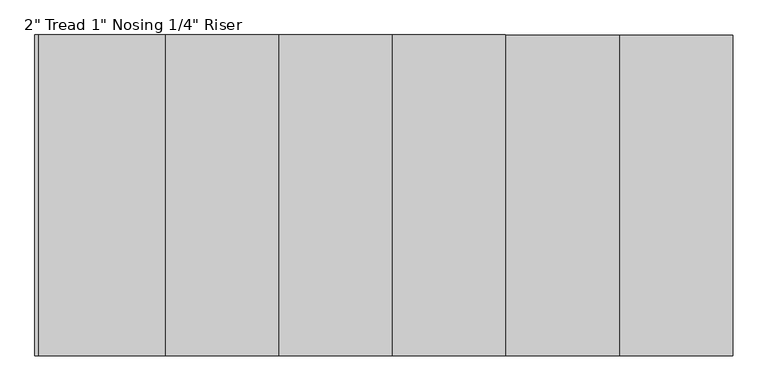
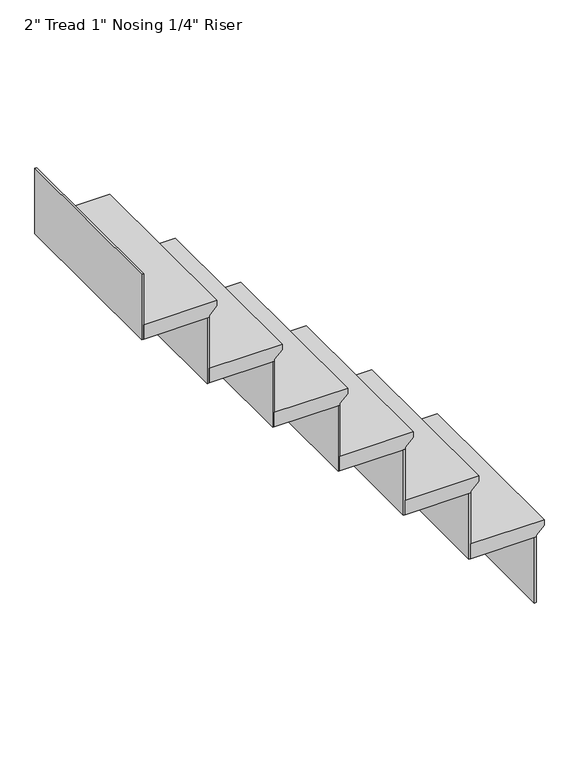
"""IFC4 building model written with IfcOpenShell, lengths in millimetres: stair flight geometry."""

from ifc_helpers import new_model, si_unit, frame, origin, place, context, project, spatial, polyline, outline, extrude, source, transform, mapped, element, save


def stair_flight_92f8819d(model_context):
    return source(origin(), model_context, "Body", "SweptSolid", [
        extrude(outline(polyline([(8229.6, -3732.7409298), (8229.6, -3974.0409298), (8178.8, -3974.0409298), (8178.8, -3758.1409298), (8185.15, -3758.1409298), (8210.55, -3732.7409298), (8229.6, -3732.7409298)])), frame((0.0, -4554.9664375, 0.0), z_axis=(0.0, 1.0, 0.0), x_axis=(0.0, 0.0, 1.0)), (0.0, 0.0, 1.0), 609.6),
        extrude(outline(polyline([(-3764.4909298, -3945.3664375), (-3758.1409298, -3945.3664375), (-3758.1409298, -4554.9664375), (-3764.4909298, -4554.9664375), (-3764.4909298, -3945.3664375)])), frame((0.0, 0.0, 7950.2), z_axis=(0.0, 0.0, 1.0), x_axis=(1.0, 0.0, 0.0)), (0.0, 0.0, 1.0), 228.6),
        extrude(outline(polyline([(-3980.3909298, -3945.3664375), (-3974.0409298, -3945.3664375), (-3974.0409298, -4554.9664375), (-3980.3909298, -4554.9664375), (-3980.3909298, -3945.3664375)])), frame((0.0, 0.0, 8178.8), z_axis=(0.0, 0.0, 1.0), x_axis=(1.0, 0.0, 0.0)), (0.0, 0.0, 1.0), 228.6),
        extrude(outline(polyline([(8458.2, -3948.6409298), (8458.2, -4189.9409298), (8407.4, -4189.9409298), (8407.4, -3974.0409298), (8413.75, -3974.0409298), (8439.15, -3948.6409298), (8458.2, -3948.6409298)])), frame((0.0, -4554.9664375, 0.0), z_axis=(0.0, 1.0, 0.0), x_axis=(0.0, 0.0, 1.0)), (0.0, 0.0, 1.0), 609.6),
        extrude(outline(polyline([(-4196.2909298, -3945.3664375), (-4189.9409298, -3945.3664375), (-4189.9409298, -4554.9664375), (-4196.2909298, -4554.9664375), (-4196.2909298, -3945.3664375)])), frame((0.0, 0.0, 8407.4), z_axis=(0.0, 0.0, 1.0), x_axis=(1.0, 0.0, 0.0)), (0.0, 0.0, 1.0), 228.6),
        extrude(outline(polyline([(8686.8, -4164.5409298), (8686.8, -4405.8409298), (8636.0, -4405.8409298), (8636.0, -4189.9409298), (8642.35, -4189.9409298), (8667.75, -4164.5409298), (8686.8, -4164.5409298)])), frame((0.0, -4554.9664375, 0.0), z_axis=(0.0, 1.0, 0.0), x_axis=(0.0, 0.0, 1.0)), (0.0, 0.0, 1.0), 609.6),
        extrude(outline(polyline([(-4412.1909298, -3945.3664375), (-4405.8409298, -3945.3664375), (-4405.8409298, -4554.9664375), (-4412.1909298, -4554.9664375), (-4412.1909298, -3945.3664375)])), frame((0.0, 0.0, 8636.0), z_axis=(0.0, 0.0, 1.0), x_axis=(1.0, 0.0, 0.0)), (0.0, 0.0, 1.0), 228.6),
        extrude(outline(polyline([(8915.4, -4380.4409298), (8915.4, -4621.7409298), (8864.6, -4621.7409298), (8864.6, -4405.8409298), (8870.95, -4405.8409298), (8896.35, -4380.4409298), (8915.4, -4380.4409298)])), frame((0.0, -4554.9664375, 0.0), z_axis=(0.0, 1.0, 0.0), x_axis=(0.0, 0.0, 1.0)), (0.0, 0.0, 1.0), 609.6),
        extrude(outline(polyline([(-4628.0909298, -3945.3664375), (-4621.7409298, -3945.3664375), (-4621.7409298, -4554.9664375), (-4628.0909298, -4554.9664375), (-4628.0909298, -3945.3664375)])), frame((0.0, 0.0, 8864.6), z_axis=(0.0, 0.0, 1.0), x_axis=(1.0, 0.0, 0.0)), (0.0, 0.0, 1.0), 228.6),
        extrude(outline(polyline([(9144.0, -4596.3409298), (9144.0, -4837.6409298), (9093.2, -4837.6409298), (9093.2, -4621.7409298), (9099.55, -4621.7409298), (9124.95, -4596.3409298), (9144.0, -4596.3409298)])), frame((0.0, -4554.9664375, 0.0), z_axis=(0.0, 1.0, 0.0), x_axis=(0.0, 0.0, 1.0)), (0.0, 0.0, 1.0), 609.6),
        extrude(outline(polyline([(-4843.9909298, -3945.3664375), (-4837.6409298, -3945.3664375), (-4837.6409298, -4554.9664375), (-4843.9909298, -4554.9664375), (-4843.9909298, -3945.3664375)])), frame((0.0, 0.0, 9093.2), z_axis=(0.0, 0.0, 1.0), x_axis=(1.0, 0.0, 0.0)), (0.0, 0.0, 1.0), 228.6),
        extrude(outline(polyline([(-5059.8909298, -3945.3664375), (-5053.5409298, -3945.3664375), (-5053.5409298, -4554.9664375), (-5059.8909298, -4554.9664375), (-5059.8909298, -3945.3664375)])), frame((0.0, 0.0, 9321.8), z_axis=(0.0, 0.0, 1.0), x_axis=(1.0, 0.0, 0.0)), (0.0, 0.0, 1.0), 228.6),
        extrude(outline(polyline([(9372.6, -4812.2409298), (9372.6, -5053.5409298), (9321.8, -5053.5409298), (9321.8, -4837.6409298), (9328.15, -4837.6409298), (9353.55, -4812.2409298), (9372.6, -4812.2409298)])), frame((0.0, -4554.9664375, 0.0), z_axis=(0.0, 1.0, 0.0), x_axis=(0.0, 0.0, 1.0)), (0.0, 0.0, 1.0), 609.6),
    ])


if __name__ == "__main__":
    model = new_model("IFC4")
    model_context = context("Model", 3, world=origin())
    ifc_project = project(units=[si_unit("LENGTHUNIT", "METRE", prefix="MILLI")], contexts=[model_context])
    site = spatial("IfcSite", under=ifc_project)
    building = spatial("IfcBuilding", under=site)
    placement = place(None, origin())
    stair_flight_shape = stair_flight_92f8819d(model_context)
    element("IfcStairFlight", 1, ObjectType="2\" Tread 1\" Nosing 1/4\" Riser", at=placement, inside=building, context=model_context, shape_type="MappedRepresentation", body=[
        mapped(stair_flight_shape, transform((0.0, 0.0, 0.0), x_axis=(1.0, 0.0, 0.0), y_axis=(0.0, 1.0, 0.0), z_axis=(0.0, 0.0, 1.0))),
    ])
    save(model, "model.ifc")
